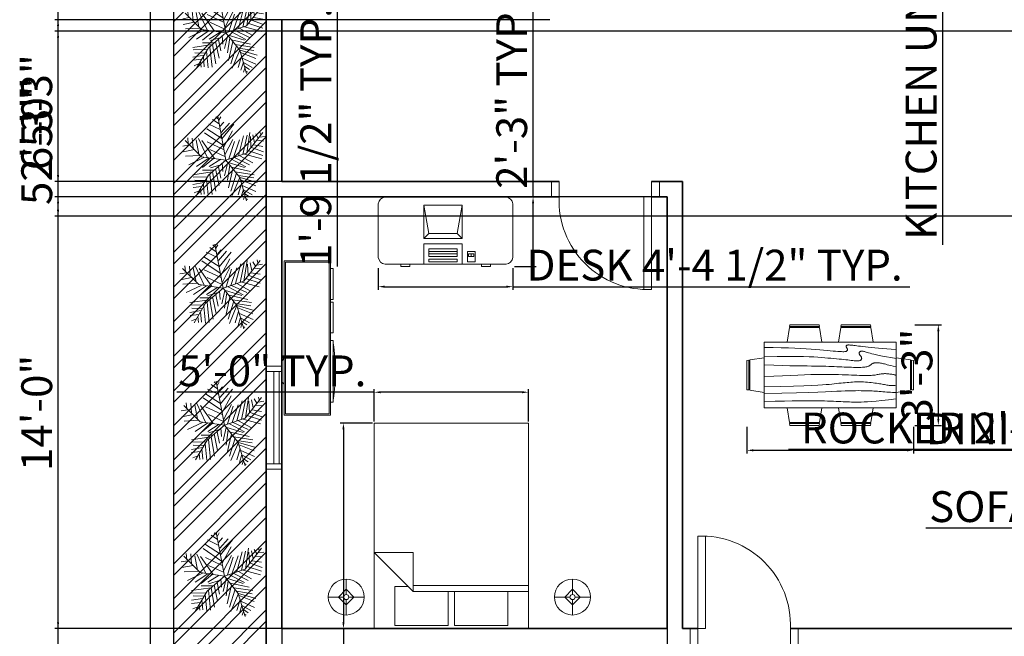
# Model space of a CAD drawing. Units: inches. Extents: x 2297 to 3143, y 440 to 1351.
# Tile 2 of 6: x 2342 to 2725, y 704 to 944. Entities that reach past the tile are written whole.
import ezdxf

# ---------------------------------------------------------------- set-up
doc = ezdxf.new("R2010")
doc.units = ezdxf.units.IN
for name, color, linetype, lineweight in [('A-ANNO-DIMS', 2, 'Continuous', 18), ('A-DOOR', 4, 'Continuous', 20), ('A-EQPM', 8, 'Continuous', 18), ('A-FURN', 8, 'Continuous', 18), ('A-GLAZ', 4, 'Continuous', 18), ('A-WALL', 7, 'Continuous', 35), ('C-PROP', 7, 'Continuous', 25), ('C-SITE-PATT', 252, 'Continuous', 13), ('E-LITE', 9, 'Continuous', 13), ('L-PLNT', 3, 'Continuous', 13)]:
    doc.layers.add(name, color=color, linetype=linetype, lineweight=lineweight)
doc.styles.get("Standard").update_dxf_attribs({"font": 'arial.ttf'})
doc.dimstyles.new('ISO-25', dxfattribs={"dimtxt": 12, "dimasz": 2.5, "dimexe": 1.25, "dimexo": 0.625, "dimtad": 1, "dimdec": 1, "dimlunit": 3, "dimtxsty": 'Standard', "dimcen": 2.5, "dimadec": 0, "dimazin": 0, "dimtfac": 1, "dimtdec": 1, "dimtmove": 0, "dimatfit": 3, "dimfxl": 1, "dimarcsym": 0})

# ---------------------------------------------------------------- blocks, each defined once
blk = doc.blocks.new('Dining Set - 36 x 72 in.')
for p, q in [((-22, 27.5), (-22.1562, 26.50042)), ((-22, 27.5), (-6, 27.5)), ((-5.8437, 26.49966), (-6, 27.5)), ((6, 27.5), (5.8438, 26.50042)), ((6, 27.5), (22, 27.5)), ((22.1563, 26.49966), (22, 27.5)), ((-22.2343, 26.00059), (-23.4847, 17.99762)), ((-22.2304, 26), (-5.7608, 26)), ((-5.8416, 26.5), (-22.1534, 26.5)), ((-4.5152, 17.99762), (-5.7655, 25.99926)), ((5.7657, 26.00059), (4.5153, 17.99762)), ((5.7696, 26), (22.2392, 26)), ((22.1584, 26.5), (5.8466, 26.5)), ((23.4848, 17.99762), (22.2345, 25.99926)), ((36, 18), (-36, 18)), ((-36, 18), (-36, -18)), ((36, -18), (36, 18)), ((-45.5, 8), (-44.5004, 8.15617)), ((-45.5, 8), (-45.5, -8)), ((-44.5, -8.15843), (-44.5, 8.15338)), ((-44.0006, 8.23428), (-35.9976, 9.48474)), ((-44, 8.23041), (-44, -8.23915)), ((44.0006, 8.23428), (35.9976, 9.48474)), ((44, 8.23041), (44, -8.23915)), ((44.5, -8.15843), (44.5, 8.15338)), ((45.5, 8), (44.5005, 8.15617)), ((45.5, 8), (45.5, -8)), ((-44.4997, -8.15631), (-45.5, -8)), ((-35.9976, -9.48476), (-43.9993, -8.2345)), ((35.9976, -9.48476), (43.9993, -8.2345)), ((44.4997, -8.15631), (45.5, -8)), ((-36, -18), (36, -18)), ((-22.2343, -26.0006), (-23.4847, -17.99762)), ((-4.5152, -17.99762), (-5.7655, -25.99928)), ((5.7657, -26.0006), (4.5153, -17.99762)), ((23.4848, -17.99762), (22.2345, -25.99928)), ((-22.2304, -26), (-5.7608, -26)), ((-22, -27.5), (-22.1562, -26.50044)), ((-5.8416, -26.5), (-22.1534, -26.5)), ((-5.8437, -26.49967), (-6, -27.5)), ((5.7696, -26), (22.2392, -26)), ((6, -27.5), (5.8438, -26.50044)), ((22.1584, -26.5), (5.8466, -26.5)), ((22.1563, -26.49967), (22, -27.5)), ((-22, -27.5), (-6, -27.5)), ((6, -27.5), (22, -27.5))]:
    blk.add_line(p, q)
for points in [[(-36, 15), (-31.1772, 14.97754), (-26.8079, 14.91406), (-22.8538, 14.81543), (-19.276, 14.6875), (-16.0362, 14.53613), (-13.0957, 14.36718), (-10.4159, 14.18652), (-7.9583, 14), (-5.6904, 13.81315), (-3.6035, 13.63021), (-1.6954, 13.45508), (0.0365, 13.29166), (1.5945, 13.14388), (2.9811, 13.01562), (4.1988, 12.9108), (5.25, 12.83333), (6.1393, 12.78613), (6.8802, 12.76823), (7.4883, 12.77767), (7.9792, 12.8125), (8.3685, 12.87077), (8.6719, 12.95052), (8.9049, 13.0498), (9.0833, 13.16666), (9.2205, 13.29899), (9.3216, 13.44401), (9.3895, 13.59879), (9.4271, 13.76041), (9.4373, 13.92594), (9.4232, 14.09245), (9.3875, 14.257), (9.3333, 14.41666), (9.2638, 14.56917), (9.1836, 14.71484), (9.0975, 14.85465), (9.0104, 14.98958), (8.9272, 15.1206), (8.8529, 15.2487), (8.7922, 15.37483), (8.75, 15.5), (8.7305, 15.62467), (8.7344, 15.74739), (8.7617, 15.86621), (8.8125, 15.97916), (8.8867, 16.08431), (8.9844, 16.17968), (9.1055, 16.26334), (9.25, 16.33333), (9.4189, 16.38802), (9.6172, 16.42708), (9.8506, 16.45052), (10.125, 16.45833), (10.4463, 16.45052), (10.8203, 16.42708), (11.2529, 16.38802), (11.75, 16.33333), (12.3184, 16.26318), (12.9694, 16.17838), (13.7151, 16.07991), (14.5677, 15.96875), (15.5395, 15.84586), (16.6426, 15.71224), (17.8893, 15.56884), (19.2917, 15.41666), (20.859, 15.25667), (22.5879, 15.08984), (24.4721, 14.91715), (26.5052, 14.73958), (28.6809, 14.5581), (30.9929, 14.3737), (33.4347, 14.18733), (36, 14)], [(-36, 10), (-28.9766, 10.14274), (-23.1725, 10.20442), (-18.4241, 10.19775), (-14.5677, 10.13541), (-11.4399, 10.03011), (-8.877, 9.89453), (-6.7154, 9.74137), (-4.7917, 9.58333), (-2.9698, 9.43082), (-1.2246, 9.28515), (0.4415, 9.14534), (2.026, 9.01041), (3.5266, 8.87939), (4.9408, 8.7513), (6.266, 8.62516), (7.5, 8.5), (8.6411, 8.37549), (9.6914, 8.2539), (10.6538, 8.13818), (11.5312, 8.03125), (12.3267, 7.93603), (13.043, 7.85547), (13.6831, 7.79248), (14.25, 7.75), (14.7471, 7.7303), (15.1797, 7.73307), (15.5537, 7.75732), (15.875, 7.80208), (16.1494, 7.86637), (16.3828, 7.94922), (16.5811, 8.04964), (16.75, 8.16666), (16.8944, 8.29915), (17.0143, 8.44531), (17.1089, 8.60319), (17.1771, 8.77083), (17.218, 8.94629), (17.2305, 9.1276), (17.2137, 9.31282), (17.1667, 9.5), (17.0895, 9.6875), (16.987, 9.875), (16.8649, 10.0625), (16.7292, 10.25), (16.5856, 10.4375), (16.4401, 10.625), (16.2985, 10.8125), (16.1667, 11), (16.05, 11.18733), (15.9518, 11.3737), (15.8752, 11.5581), (15.8229, 11.73958), (15.798, 11.91715), (15.8034, 12.08984), (15.842, 12.25667), (15.9167, 12.41666), (16.0295, 12.56836), (16.1784, 12.70833), (16.3605, 12.83268), (16.5729, 12.9375), (16.8127, 13.01888), (17.0768, 13.07291), (17.3625, 13.0957), (17.6667, 13.08333), (17.9894, 13.03312), (18.3418, 12.94726), (18.7382, 12.82918), (19.1927, 12.68229), (19.7195, 12.51001), (20.3327, 12.31575), (21.0465, 12.10294), (21.875, 11.875), (22.8357, 11.63354), (23.959, 11.37304), (25.2786, 11.08618), (26.8282, 10.76562), (28.6414, 10.40405), (30.752, 9.99414), (33.1936, 9.52856), (36, 9)], [(-36, 5.5), (-30.7157, 5.3348), (-26.069, 5.20963), (-21.9946, 5.11767), (-18.4271, 5.05208), (-15.3009, 5.00602), (-12.5508, 4.97265), (-10.1112, 4.94515), (-7.9167, 4.91666), (-5.909, 4.88167), (-4.0586, 4.83984), (-2.3429, 4.79215), (-0.7396, 4.73958), (0.7739, 4.6831), (2.22, 4.6237), (3.6213, 4.56233), (5, 4.5), (6.373, 4.43782), (7.7344, 4.3776), (9.0723, 4.32129), (10.375, 4.27083), (11.6309, 4.22819), (12.8281, 4.19531), (13.9551, 4.17415), (15, 4.16666), (15.954, 4.17448), (16.819, 4.19791), (17.6001, 4.23698), (18.3021, 4.29166), (18.9299, 4.36198), (19.4883, 4.44791), (19.9823, 4.54948), (20.4167, 4.66666), (20.7969, 4.79899), (21.1302, 4.94401), (21.4245, 5.09879), (21.6875, 5.26041), (21.9271, 5.42594), (22.1511, 5.59245), (22.3672, 5.757), (22.5834, 5.91666), (22.8065, 6.06868), (23.0404, 6.21093), (23.2879, 6.34147), (23.5521, 6.45833), (23.8358, 6.55957), (24.142, 6.64323), (24.4735, 6.70735), (24.8334, 6.75), (25.2235, 6.76969), (25.642, 6.76692), (26.0858, 6.74267), (26.5521, 6.69791), (27.0379, 6.63362), (27.5404, 6.55078), (28.0565, 6.45036), (28.5834, 6.33333), (29.1242, 6.19987), (29.7071, 6.04687), (30.3661, 5.87044), (31.1354, 5.66666), (32.0493, 5.43164), (33.142, 5.16146), (34.4475, 4.85221), (36, 4.5)], [(-36, -1), (-30.7915, -0.6591), (-26.0195, -0.38216), (-21.6519, -0.16284), (-17.6563, 0.00521), (-14.0005, 0.12833), (-10.6523, 0.21289), (-7.5796, 0.26522), (-4.75, 0.29166), (-2.134, 0.29793), (0.2878, 0.28711), (2.5317, 0.26163), (4.6146, 0.22396), (6.5529, 0.17651), (8.3633, 0.12174), (10.0623, 0.06209), (11.6667, 0), (13.1899, -0.06201), (14.6341, -0.1211), (15.9982, -0.17432), (17.2813, -0.21875), (18.4823, -0.25147), (19.6003, -0.26953), (20.6343, -0.27002), (21.5834, -0.25), (22.4481, -0.20768), (23.2357, -0.14584), (23.9549, -0.06836), (24.6146, 0.02083), (25.2235, 0.11784), (25.7904, 0.21875), (26.3241, 0.31966), (26.8334, 0.41666), (27.3265, 0.50618), (27.8099, 0.58593), (28.2894, 0.65397), (28.7709, 0.70833), (29.2601, 0.74707), (29.763, 0.76823), (30.2855, 0.76985), (30.8334, 0.75), (31.4088, 0.70784), (31.9994, 0.64713), (32.589, 0.57275), (33.1615, 0.48958), (33.7008, 0.4025), (34.1908, 0.3164), (34.6153, 0.23616), (34.9584, 0.16666), (35.2099, 0.11165), (35.3848, 0.07031), (35.504, 0.04069), (35.5886, 0.02083), (35.6594, 0.00879), (35.7377, 0.0026), (35.8442, 0.00032), (36, 0)], [(-36, -6.5), (-27.1843, -6.31267), (-20.084, -6.1263), (-14.469, -5.9419), (-10.1094, -5.76042), (-6.7752, -5.58285), (-4.2363, -5.41016), (-2.2629, -5.24333), (-0.625, -5.08334), (0.8708, -4.93099), (2.2715, -4.78646), (3.5872, -4.64974), (4.8281, -4.52084), (6.0046, -4.39974), (7.127, -4.28646), (8.2053, -4.18099), (9.25, -4.08334), (10.2705, -3.99382), (11.2734, -3.91407), (12.2647, -3.84603), (13.25, -3.79167), (14.2354, -3.75293), (15.2266, -3.73177), (16.2295, -3.73015), (17.25, -3.75), (18.2912, -3.79248), (19.3451, -3.85547), (20.4009, -3.93604), (21.4479, -4.03125), (22.4754, -4.13819), (23.4727, -4.25391), (24.4289, -4.37549), (25.3334, -4.5), (26.1785, -4.62492), (26.9694, -4.74935), (27.7145, -4.87281), (28.4219, -4.99479), (29.1, -5.11483), (29.7572, -5.23242), (30.4016, -5.34709), (31.0417, -5.45834), (31.6837, -5.56437), (32.3262, -5.65821), (32.9658, -5.73153), (33.599, -5.77604), (34.2224, -5.78345), (34.8327, -5.74545), (35.4264, -5.65373), (36, -5.5)], [(-36, -10), (-26.4022, -9.81299), (-18.4675, -9.62891), (-11.9839, -9.45069), (-6.7396, -9.28125), (-2.5226, -9.12354), (0.8789, -8.98047), (3.6769, -8.85498), (6.0833, -8.75), (8.2767, -8.66765), (10.3021, -8.60677), (12.1712, -8.56543), (13.8958, -8.54167), (15.4876, -8.53353), (16.9583, -8.53907), (18.3197, -8.55632), (19.5834, -8.58334), (20.7616, -8.61841), (21.8685, -8.66081), (22.9188, -8.71004), (23.9271, -8.76563), (24.9081, -8.82707), (25.8763, -8.89388), (26.8465, -8.96558), (27.8334, -9.04167), (28.8474, -9.12118), (29.8828, -9.20117), (30.93, -9.27824), (31.9792, -9.34896), (33.0205, -9.40991), (34.0443, -9.45768), (35.0407, -9.48885), (36, -9.5)], [(-36, -14.5), (-30.0881, -14.33513), (-25.0332, -14.21224), (-20.7312, -14.12647), (-17.0781, -14.07292), (-13.97, -14.04671), (-11.3027, -14.04297), (-8.9724, -14.05681), (-6.875, -14.08334), (-4.9224, -14.11833), (-3.0905, -14.16016), (-1.3709, -14.20785), (0.2448, -14.26042), (1.7647, -14.3169), (3.1973, -14.3763), (4.5507, -14.43767), (5.8333, -14.5), (7.0554, -14.5621), (8.235, -14.62175), (9.3922, -14.67652), (10.5469, -14.72396), (11.7192, -14.76164), (12.929, -14.78711), (14.1965, -14.79794), (15.5417, -14.79167), (16.9933, -14.76424), (18.6152, -14.70508), (20.4804, -14.60197), (22.6615, -14.44271), (25.2312, -14.21509), (28.2624, -13.9069), (31.8277, -13.50594), (36, -13)]]:
    blk.add_lwpolyline(points)
blk = doc.blocks.new('Bed - Queen')
for p, q in [((0, -80.00003), (0, 0)), ((0, 0), (59.99999, 0)), ((59.99999, 0), (59.99999, -80.00003)), ((7.99999, -1.2), (28.79998, -1.2)), ((7.99999, -14.4), (7.99999, -1.2)), ((28.79998, -1.2), (28.79998, -14.4)), ((31.19999, -1.2), (51.99999, -1.2)), ((31.19999, -14.4), (31.19999, -1.2)), ((51.99999, -1.2), (51.99999, -16.4)), ((0, -14.4), (44.8, -14.4)), ((59.99999, -29.6), (44.8, -14.4)), ((44.8, -14.4), (44.8, -29.6)), ((44.8, -16.8), (0, -16.8)), ((51.99999, -16.4), (46.79936, -16.4)), ((44.8, -29.6), (59.99999, -29.6)), ((59.99999, -80.00003), (0, -80.00003))]:
    blk.add_line(p, q)
blk = doc.blocks.new('*U16')
for p, q in [((-8.737, 47.138), (-17.069, 52.711)), ((-10.186, 53.64), (-13.084, 55.962)), ((0, 0), (-10.5, 57)), ((-9.099, 51.782), (-6.563, 55.962)), ((-5.114, 28.097), (-24.676, 40.636)), ((-7.288, 39.707), (-21.778, 46.673)), ((-7.65, 43.423), (-2.578, 49.46)), ((-5.839, 35.992), (4.667, 48.067)), ((-5.114, 27.632), (10.463, 46.673)), ((-48.585, 21.131), (-49.309, 29.026)), ((-43.513, 28.561), (-42.427, 15.558)), ((-38.442, 26.239), (-34.819, 7.663)), ((-35.544, 28.097), (-24.314, 3.947)), ((-3.665, 19.273), (-27.574, 35.527)), ((-2.941, 16.486), (8.652, 37.85)), ((-1.129, 6.734), (9.014, 26.704)), ((10.101, 3.483), (17.708, 26.239)), ((16.259, 5.805), (23.142, 31.348)), ((22.055, 7.198), (27.489, 32.277)), ((27, 9), (48, 36)), ((27.127, 9.056), (31.112, 35.992)), ((31.836, 30.883), (32.561, 16.486)), ((35.096, 32.741), (37.27, 22.524)), ((38.719, 34.134), (41.979, 28.561)), ((40.53, 25.775), (48.862, 24.846)), ((43.791, 29.954), (51.036, 30.883)), ((44.153, 36.456), (45.239, 32.741)), ((-47.498, 19.737), (-55.83, 18.344)), ((-40.615, 13.7), (-55.105, 10.913)), ((-31.5, 4.5), (-52.5, 25.5)), ((-14.533, 2.09), (-30.834, 25.31)), ((-24.314, 23.917), (-2.941, 13.7)), ((-20.691, 13.7), (-1.129, 4.876)), ((3.942, 1.625), (11.187, 24.381)), ((33.285, 16.486), (48.862, 10.913)), ((36.183, 19.737), (48.137, 17.88)), ((-33.37, 6.269), (-52.207, 5.34)), ((-28.299, 3.483), (-47.86, -5.805)), ((-21.416, 3.018), (-38.079, -8.128)), ((0, 0), (-31.5, 4.5)), ((-15.982, 2.09), (-30.11, -9.521)), ((0, 0), (-22.5, -19.5)), ((-6.563, 1.161), (-21.416, -8.128)), ((0, 0), (27, 9)), ((0, 0), (18, -22.5)), ((6.478, 1.625), (26.04, -8.592)), ((11.187, 3.483), (30.749, -5.805)), ((18.07, 5.805), (35.096, -3.483)), ((24.229, 7.663), (46.688, 1.625)), ((29.662, 12.307), (48.137, 6.269)), ((-6.563, -5.805), (-19.967, -9.985)), ((-13.446, -11.378), (-8.737, -32.741)), ((-9.461, -8.592), (-6.201, -23.453)), ((-4.752, -3.483), (-3.665, -14.629)), ((2.493, -3.019), (-1.491, -20.202)), ((1.769, -2.555), (24.229, -9.521)), ((5.029, -6.27), (2.131, -25.775)), ((9.014, -11.378), (3.58, -35.992)), ((7.565, -9.056), (32.198, -14.629)), ((-17.431, -15.094), (-42.789, -18.809)), ((-24.314, -21.596), (-42.427, -22.06)), ((-22.5, -19.5), (-37.5, -45)), ((-15.257, -12.772), (-30.11, -12.772)), ((-25.038, -23.918), (-22.865, -45.281)), ((-20.691, -18.345), (-17.793, -44.352)), ((-17.069, -15.094), (-12.721, -40.172)), ((14.085, -16.951), (6.478, -40.172)), ((18.07, -22.524), (8.289, -45.745)), ((12.274, -15.094), (36.907, -18.809)), ((16.259, -19.738), (36.183, -22.989)), ((18, -22.5), (27, -52.5)), ((18.433, -22.524), (40.53, -29.026)), ((19.157, -25.311), (38.719, -33.206)), ((-28.299, -29.026), (-42.789, -31.348)), ((-30.834, -34.135), (-42.427, -35.528)), ((-26.849, -26.24), (-40.253, -25.775)), ((-32.646, -36.921), (-31.921, -44.352)), ((-29.023, -30.884), (-27.936, -43.887)), ((20.244, -30.419), (15.897, -44.816)), ((22.78, -37.85), (19.519, -48.532)), ((21.331, -32.741), (39.081, -40.636)), ((-34.457, -39.708), (-40.978, -42.494)), ((22.78, -38.314), (34.372, -44.816)), ((24.591, -45.745), (23.142, -50.854)), ((24.591, -43.423), (30.749, -47.603)), ((26.764, -49.925), (28.213, -50.854))]:
    blk.add_line(p, q)
blk = doc.blocks.new('Lamp - Table')
for p, q in [((0, 7), (0, 1)), ((-1, 0), (-7, 0)), ((0, 3), (-3, 0)), ((-3, 0), (0, -3)), ((3, 0), (0, 3)), ((0, -3), (3, 0)), ((1, 0), (7, 0)), ((0, -1), (0, -7))]:
    blk.add_line(p, q)
for radius in [7, 1]:
    blk.add_circle((0, 0), radius)
blk = doc.blocks.new('Desk - 30 x 60 in.')
for p, q in [((-26.999995, 0), (26.999995, 0)), ((-29.999995, -27), (-29.999995, -3)), ((29.999995, -3), (29.999995, -27)), ((26.999995, -30), (-26.999995, -30)), ((-20.000005, -30), (-20.000005, -31)), ((-16.000005, -31), (-16.000005, -30)), ((15.999995, -31), (15.999995, -30)), ((19.999995, -30), (19.999995, -31)), ((-20.000005, -31), (-16.000005, -31)), ((19.999995, -31), (15.999995, -31))]:
    blk.add_line(p, q)
for centre, start, end in [((-26.499995, -3.5), 98.1301, 171.8699), ((26.499995, -3.5), 8.130102, 81.8699), ((-26.499995, -26.5), 188.1301, 261.8699), ((26.499995, -26.5), 278.1301, 351.8699)]:
    blk.add_arc(centre, 3.535534, start, end)
blk = doc.blocks.new('Computer Terminal')
for p, q in [((-10, 11.5), (5, 11.5)), ((-8, 0.5), (-10, 11.5)), ((-10, -1.5), (-10, 11.5)), ((5, 11.5), (3, 0.5)), ((5, 11.5), (5, -1.5)), ((-10, -1.5), (-8, 0.5)), ((3, 0.5), (-8, 0.5)), ((3, 0.5), (5, -1.5)), ((5, -1.5), (-10, -1.5)), ((-10, -11.5), (-10, -3.5)), ((-10, -3.5), (5, -3.5)), ((5, -3.5), (5, -11.5)), ((-8, -5.5), (-8, -8.5)), ((3, -5.5), (-8, -5.5)), ((3, -6.5), (-8, -6.5)), ((-8, -7.5), (3, -7.5)), ((3, -8.5), (3, -5.5)), ((10, -6.5), (7, -6.5)), ((7, -6.5), (7, -10.5)), ((9.5, -7.5), (7.5, -7.5)), ((7.5, -7.5), (7.5, -8.5)), ((8.5, -7.5), (8.5, -8.5)), ((9.5, -8.5), (9.5, -7.5)), ((10, -10.5), (10, -6.5)), ((-8, -8.5), (3, -8.5)), ((-8, -9.5), (-8, -10.5)), ((3, -9.5), (-8, -9.5)), ((-8, -10.5), (3, -10.5)), ((3, -10.5), (3, -9.5)), ((7, -10.5), (10, -10.5)), ((7.5, -8.5), (9.5, -8.5)), ((5, -11.5), (-10, -11.5))]:
    blk.add_line(p, q)
blk = doc.blocks.new('Entertainment Center')
for p, q in [((-4, 0), (-5, -1)), ((4, 0), (-4, 0)), ((5, -1), (4, 0)), ((-17, -19), (-17, -1)), ((-17, -1), (43, -1)), ((-16.5, -18.5), (-16.5, -1.5)), ((-16.5, -1.5), (42.5, -1.5)), ((42.5, -1.5), (42.5, -18.5)), ((43, -1), (43, -19)), ((43, -19), (-17, -19)), ((42.5, -18.5), (-16.5, -18.5)), ((-12, -20), (-12, -19)), ((12, -19), (12, -20)), ((15, -20), (15, -19)), ((27, -19), (27, -20)), ((28, -20), (28, -19)), ((40, -19), (40, -20)), ((12, -20), (-12, -20)), ((27, -20), (15, -20)), ((40, -20), (28, -20))]:
    blk.add_line(p, q)
blk.add_arc((0, 40), 61, 259.6111, 280.3889)
blk = doc.blocks.new('DOOR-36IN-6IN-JAMB')
for p, q in [((0, 6), (0, 0)), ((3, 6), (3, 0)), ((39, 6), (39, 0)), ((42, 6), (42, 0))]:
    blk.add_line(p, q)
blk.add_lwpolyline([(39, 6), (36, 6), (36, 42), (39, 42)], close=True)
blk.add_arc((37.5, 7.5), 34.53, 87.5104, 182.4896)
blk = doc.blocks.new('WIN-36IN-6IN-WALL')
for p, q in [((6, 40), (0, 40)), ((6, 38), (0, 38)), ((3, 38), (3, 2)), ((5, 38), (5, 2)), ((0, 2), (6, 2)), ((0, 0), (6, 0))]:
    blk.add_line(p, q)
blk = doc.blocks.new('*D33')
at = {"layer": 'A-ANNO-DIMS', "color": 0, "lineweight": -2, "transparency": 16777216}
for p, q in [((2481.79, 846.95), (2481.79, 838.47)), ((2534.17, 846.95), (2534.17, 838.47)), ((2484.29, 839.72), (2531.67, 839.72)), ((2534.17, 839.72), (2688.74, 839.72))]:
    blk.add_line(p, q, dxfattribs=at)
at = {"layer": 'A-ANNO-DIMS', "color": 0, "transparency": 16777216}
for points in [[(2484.29, 840.13), (2484.29, 839.3), (2481.79, 839.72)], [(2531.67, 840.13), (2531.67, 839.3), (2534.17, 839.72)]]:
    blk.add_solid(points, dxfattribs=at)
at = {"layer": 'Defpoints', "color": 0, "transparency": 16777216}
for p in [(2481.79, 847.57), (2534.17, 847.57), (2534.17, 839.72)]:
    blk.add_point(p, dxfattribs=at)
at = {"layer": 'A-ANNO-DIMS', "color": 0, "transparency": 16777216, "insert": (2612.7, 846.55), "char_height": 12, "attachment_point": 5}
blk.add_mtext('DESK 4\'-4 1/2" TYP.', dxfattribs=at)
blk = doc.blocks.new('*D34')
at = {"layer": 'A-ANNO-DIMS', "color": 0, "lineweight": -2, "transparency": 16777216}
for p, q in [((2542.03, 874.63), (2542.03, 951.74)), ((2534.79, 874.63), (2543.28, 874.63)), ((2542.03, 850.07), (2542.03, 872.13)), ((2534.79, 847.57), (2543.28, 847.57))]:
    blk.add_line(p, q, dxfattribs=at)
at = {"layer": 'A-ANNO-DIMS', "color": 0, "transparency": 16777216}
for points in [[(2541.61, 872.13), (2542.44, 872.13), (2542.03, 874.63)], [(2541.61, 850.07), (2542.44, 850.07), (2542.03, 847.57)]]:
    blk.add_solid(points, dxfattribs=at)
at = {"layer": 'Defpoints', "color": 0, "transparency": 16777216}
for p in [(2534.17, 874.63), (2542.03, 874.63), (2534.17, 847.57)]:
    blk.add_point(p, dxfattribs=at)
at = {"layer": 'A-ANNO-DIMS', "color": 0, "transparency": 16777216, "insert": (2535.27, 914.43), "char_height": 12, "attachment_point": 5, "rotation": 90}
blk.add_mtext('2\'-3" TYP.', dxfattribs=at)
blk = doc.blocks.new('*D37')
at = {"layer": 'A-ANNO-DIMS', "color": 0, "lineweight": -2, "transparency": 16777216}
for p, q in [((2479.6, 786.63), (2466.97, 786.63)), ((2468.22, 784.13), (2468.22, 709.13)), ((2479.6, 706.63), (2466.97, 706.63)), ((2468.22, 706.63), (2468.22, 526.36))]:
    blk.add_line(p, q, dxfattribs=at)
at = {"layer": 'A-ANNO-DIMS', "color": 0, "transparency": 16777216}
for points in [[(2467.8, 784.13), (2468.64, 784.13), (2468.22, 786.63)], [(2467.8, 709.13), (2468.64, 709.13), (2468.22, 706.63)]]:
    blk.add_solid(points, dxfattribs=at)
at = {"layer": 'Defpoints', "color": 0, "transparency": 16777216}
for p in [(2480.22, 786.63), (2468.22, 706.63), (2480.22, 706.63)]:
    blk.add_point(p, dxfattribs=at)
at = {"layer": 'A-ANNO-DIMS', "color": 0, "transparency": 16777216, "insert": (2461.02, 615.25), "char_height": 12, "attachment_point": 5, "rotation": 90}
blk.add_mtext('QUEEN BED 6\'-8" TYP.', dxfattribs=at)
blk = doc.blocks.new('*D38')
at = {"layer": 'A-ANNO-DIMS', "color": 0, "lineweight": -2, "transparency": 16777216}
for p, q in [((2480.22, 798.63), (2403.32, 798.63)), ((2480.22, 787.26), (2480.22, 799.88)), ((2537.72, 798.63), (2482.72, 798.63)), ((2540.22, 787.26), (2540.22, 799.88))]:
    blk.add_line(p, q, dxfattribs=at)
at = {"layer": 'A-ANNO-DIMS', "color": 0, "transparency": 16777216}
for points in [[(2482.72, 799.05), (2482.72, 798.22), (2480.22, 798.63)], [(2537.72, 799.05), (2537.72, 798.22), (2540.22, 798.63)]]:
    blk.add_solid(points, dxfattribs=at)
at = {"layer": 'Defpoints', "color": 0, "transparency": 16777216}
for p in [(2480.22, 798.63), (2480.22, 786.63), (2540.22, 786.63)]:
    blk.add_point(p, dxfattribs=at)
at = {"layer": 'A-ANNO-DIMS', "color": 0, "transparency": 16777216, "insert": (2440.52, 805.39), "char_height": 12, "attachment_point": 5}
blk.add_mtext('5\'-0" TYP.', dxfattribs=at)
blk = doc.blocks.new('*D42')
at = {"layer": 'A-ANNO-DIMS', "color": 0, "lineweight": -2, "transparency": 16777216}
for p, q in [((2474.21, 972.57), (2464.59, 972.57)), ((2465.84, 970.07), (2465.84, 953.74)), ((2474.21, 951.24), (2464.59, 951.24)), ((2465.84, 951.24), (2465.84, 847.51))]:
    blk.add_line(p, q, dxfattribs=at)
at = {"layer": 'A-ANNO-DIMS', "color": 0, "transparency": 16777216}
for points in [[(2465.42, 970.07), (2466.25, 970.07), (2465.84, 972.57)], [(2465.42, 953.74), (2466.25, 953.74), (2465.84, 951.24)]]:
    blk.add_solid(points, dxfattribs=at)
at = {"layer": 'Defpoints', "color": 0, "transparency": 16777216}
for p in [(2474.84, 972.57), (2465.84, 951.24), (2474.84, 951.24)]:
    blk.add_point(p, dxfattribs=at)
at = {"layer": 'A-ANNO-DIMS', "color": 0, "transparency": 16777216, "insert": (2459.01, 898.13), "char_height": 12, "attachment_point": 5, "rotation": 90}
blk.add_mtext('1\'-9 1/2" TYP.', dxfattribs=at)
blk = doc.blocks.new('*D49')
at = {"layer": 'A-ANNO-DIMS', "color": 0, "lineweight": -2, "transparency": 16777216}
for p, q in [((2818.08, 745.72), (2694.9, 745.72)), ((2818.08, 735.78), (2818.08, 746.97)), ((2886.03, 745.72), (2820.58, 745.72)), ((2888.53, 735.78), (2888.53, 746.97))]:
    blk.add_line(p, q, dxfattribs=at)
at = {"layer": 'A-ANNO-DIMS', "color": 0, "transparency": 16777216}
for points in [[(2820.58, 746.14), (2820.58, 745.3), (2818.08, 745.72)], [(2886.03, 746.14), (2886.03, 745.3), (2888.53, 745.72)]]:
    blk.add_solid(points, dxfattribs=at)
at = {"layer": 'Defpoints', "color": 0, "transparency": 16777216}
for p in [(2818.08, 745.72), (2818.08, 735.15), (2888.53, 735.15)]:
    blk.add_point(p, dxfattribs=at)
at = {"layer": 'A-ANNO-DIMS', "color": 0, "transparency": 16777216, "insert": (2755.24, 752.55), "char_height": 12, "attachment_point": 5}
blk.add_mtext('SOFA 5\'-10 1/2"', dxfattribs=at)
blk = doc.blocks.new('*D53')
at = {"layer": 'A-ANNO-DIMS', "color": 0, "lineweight": -2, "transparency": 16777216}
for p, q in [((2794.15, 776.31), (2641.5, 776.31)), ((2794.15, 772.88), (2794.15, 777.56)), ((2818.65, 776.31), (2796.65, 776.31)), ((2821.15, 772.88), (2821.15, 777.56))]:
    blk.add_line(p, q, dxfattribs=at)
at = {"layer": 'A-ANNO-DIMS', "color": 0, "transparency": 16777216}
for points in [[(2796.65, 776.72), (2796.65, 775.89), (2794.15, 776.31)], [(2818.65, 776.72), (2818.65, 775.89), (2821.15, 776.31)]]:
    blk.add_solid(points, dxfattribs=at)
at = {"layer": 'Defpoints', "color": 0, "transparency": 16777216}
for p in [(2794.15, 776.31), (2794.15, 772.26), (2821.15, 772.26)]:
    blk.add_point(p, dxfattribs=at)
at = {"layer": 'A-ANNO-DIMS', "color": 0, "transparency": 16777216, "insert": (2716.58, 783.14), "char_height": 12, "attachment_point": 5}
blk.add_mtext('ROCKER 2\'-3" TYP.', dxfattribs=at)
blk = doc.blocks.new('*D61')
at = {"layer": 'A-ANNO-DIMS', "color": 0, "lineweight": -2, "transparency": 16777216}
for p, q in [((2710.47, 1077.25), (2700.22, 1077.25)), ((2701.47, 1074.75), (2701.47, 1015.6)), ((2710.47, 1013.1), (2700.22, 1013.1)), ((2701.47, 1013.1), (2701.47, 855.98))]:
    blk.add_line(p, q, dxfattribs=at)
at = {"layer": 'A-ANNO-DIMS', "color": 0, "transparency": 16777216}
for points in [[(2701.05, 1074.75), (2701.89, 1074.75), (2701.47, 1077.25)], [(2701.05, 1015.6), (2701.89, 1015.6), (2701.47, 1013.1)]]:
    blk.add_solid(points, dxfattribs=at)
at = {"layer": 'Defpoints', "color": 0, "transparency": 16777216}
for p in [(2711.09, 1077.25), (2701.47, 1013.1), (2711.09, 1013.1)]:
    blk.add_point(p, dxfattribs=at)
at = {"layer": 'A-ANNO-DIMS', "color": 0, "transparency": 16777216, "insert": (2694.64, 933.29), "char_height": 12, "attachment_point": 5, "rotation": 90}
blk.add_mtext('KITCHEN UNIT 5\'-4"', dxfattribs=at)
blk = doc.blocks.new('*D63')
at = {"layer": 'A-ANNO-DIMS', "color": 0, "lineweight": -2, "transparency": 16777216}
for p, q in [((2625.28, 785.11), (2625.28, 774.77)), ((2690.07, 785.11), (2690.07, 774.77)), ((2627.78, 776.02), (2687.57, 776.02)), ((2690.07, 776.02), (2825.72, 776.02))]:
    blk.add_line(p, q, dxfattribs=at)
at = {"layer": 'A-ANNO-DIMS', "color": 0, "transparency": 16777216}
for points in [[(2627.78, 776.44), (2627.78, 775.6), (2625.28, 776.02)], [(2687.57, 776.44), (2687.57, 775.6), (2690.07, 776.02)]]:
    blk.add_solid(points, dxfattribs=at)
at = {"layer": 'Defpoints', "color": 0, "transparency": 16777216}
for p in [(2625.28, 785.74), (2690.07, 785.74), (2690.07, 776.02)]:
    blk.add_point(p, dxfattribs=at)
at = {"layer": 'A-ANNO-DIMS', "color": 0, "transparency": 16777216, "insert": (2759.14, 782.85), "char_height": 12, "attachment_point": 5}
blk.add_mtext('DINING SET 5\'-5"', dxfattribs=at)
blk = doc.blocks.new('*D64')
at = {"layer": 'A-ANNO-DIMS', "color": 0, "lineweight": -2, "transparency": 16777216}
for p, q in [((2690.7, 824.9), (2701.04, 824.9)), ((2699.79, 788.24), (2699.79, 822.4)), ((2690.7, 785.74), (2701.04, 785.74))]:
    blk.add_line(p, q, dxfattribs=at)
at = {"layer": 'A-ANNO-DIMS', "color": 0, "transparency": 16777216}
for points in [[(2699.37, 822.4), (2700.21, 822.4), (2699.79, 824.9)], [(2699.37, 788.24), (2700.21, 788.24), (2699.79, 785.74)]]:
    blk.add_solid(points, dxfattribs=at)
at = {"layer": 'Defpoints', "color": 0, "transparency": 16777216}
for p in [(2690.07, 824.9), (2699.79, 824.9), (2690.07, 785.74)]:
    blk.add_point(p, dxfattribs=at)
at = {"layer": 'A-ANNO-DIMS', "color": 0, "transparency": 16777216, "insert": (2693.03, 805.32), "char_height": 12, "attachment_point": 5, "rotation": 90}
blk.add_mtext('3\'-3"', dxfattribs=at)
blk = doc.blocks.new('*D70')
at = {"layer": 'A-ANNO-DIMS', "color": 0, "lineweight": -2, "transparency": 16777216}
for p, q in [((2392.57, 1207.63), (2355.89, 1207.63)), ((2357.14, 583.13), (2357.14, 1205.13)), ((2437.57, 580.63), (2355.89, 580.63))]:
    blk.add_line(p, q, dxfattribs=at)
at = {"layer": 'A-ANNO-DIMS', "color": 0, "transparency": 16777216}
for points in [[(2356.73, 1205.13), (2357.56, 1205.13), (2357.14, 1207.63)], [(2356.73, 583.13), (2357.56, 583.13), (2357.14, 580.63)]]:
    blk.add_solid(points, dxfattribs=at)
at = {"layer": 'Defpoints', "color": 0, "transparency": 16777216}
for p in [(2357.14, 1207.63), (2393.19, 1207.63), (2438.19, 580.63)]:
    blk.add_point(p, dxfattribs=at)
at = {"layer": 'A-ANNO-DIMS', "color": 0, "transparency": 16777216, "insert": (2350.39, 894.13), "char_height": 12, "attachment_point": 5, "rotation": 90}
blk.add_mtext('52\'-3"', dxfattribs=at)
blk = doc.blocks.new('*D76')
at = {"layer": 'A-ANNO-DIMS', "color": 0, "lineweight": -2, "transparency": 16777216}
for p, q in [((2593.57, 874.63), (2355.89, 874.63)), ((2357.14, 709.13), (2357.14, 872.13)), ((2593.57, 706.63), (2355.89, 706.63))]:
    blk.add_line(p, q, dxfattribs=at)
at = {"layer": 'A-ANNO-DIMS', "color": 0, "transparency": 16777216}
for points in [[(2356.73, 872.13), (2357.56, 872.13), (2357.14, 874.63)], [(2356.73, 709.13), (2357.56, 709.13), (2357.14, 706.63)]]:
    blk.add_solid(points, dxfattribs=at)
at = {"layer": 'Defpoints', "color": 0, "transparency": 16777216}
for p in [(2357.14, 874.63), (2594.19, 874.63), (2594.19, 706.63)]:
    blk.add_point(p, dxfattribs=at)
at = {"layer": 'A-ANNO-DIMS', "color": 0, "transparency": 16777216, "insert": (2350.39, 790.63), "char_height": 12, "attachment_point": 5, "rotation": 90}
blk.add_mtext('14\'-0"', dxfattribs=at)
blk = doc.blocks.new('*D77')
at = {"layer": 'A-ANNO-DIMS', "color": 0, "lineweight": -2, "transparency": 16777216}
for p, q in [((2444.19, 874.01), (2444.19, 510.33)), ((2594.19, 874.01), (2594.19, 510.33)), ((2446.69, 511.58), (2591.69, 511.58))]:
    blk.add_line(p, q, dxfattribs=at)
at = {"layer": 'A-ANNO-DIMS', "color": 0, "transparency": 16777216}
for points in [[(2446.69, 512), (2446.69, 511.17), (2444.19, 511.58)], [(2591.69, 512), (2591.69, 511.17), (2594.19, 511.58)]]:
    blk.add_solid(points, dxfattribs=at)
at = {"layer": 'Defpoints', "color": 0, "transparency": 16777216}
for p in [(2444.19, 874.63), (2594.19, 874.63), (2594.19, 511.58)]:
    blk.add_point(p, dxfattribs=at)
at = {"layer": 'A-ANNO-DIMS', "color": 0, "transparency": 16777216, "insert": (2519.19, 518.34), "char_height": 12, "attachment_point": 5}
blk.add_mtext('12\'-6"', dxfattribs=at)
blk = doc.blocks.new('*D78')
at = {"layer": 'A-ANNO-DIMS', "color": 0, "lineweight": -2, "transparency": 16777216}
for p, q in [((2548.57, 943.63), (2355.89, 943.63)), ((2357.14, 883.13), (2357.14, 941.13)), ((2548.57, 880.63), (2355.89, 880.63))]:
    blk.add_line(p, q, dxfattribs=at)
at = {"layer": 'A-ANNO-DIMS', "color": 0, "transparency": 16777216}
for points in [[(2356.73, 941.13), (2357.56, 941.13), (2357.14, 943.63)], [(2356.73, 883.13), (2357.56, 883.13), (2357.14, 880.63)]]:
    blk.add_solid(points, dxfattribs=at)
at = {"layer": 'Defpoints', "color": 0, "transparency": 16777216}
for p in [(2357.14, 943.63), (2549.19, 943.63), (2549.19, 880.63)]:
    blk.add_point(p, dxfattribs=at)
at = {"layer": 'A-ANNO-DIMS', "color": 0, "transparency": 16777216, "insert": (2350.39, 912.13), "char_height": 12, "attachment_point": 5, "rotation": 90}
blk.add_mtext('5\'-3"', dxfattribs=at)
blk = doc.blocks.new('*D80')
at = {"layer": 'A-ANNO-DIMS', "color": 0, "lineweight": -2, "transparency": 16777216}
for p, q in [((2805.07, 939.13), (2355.89, 939.13)), ((2357.14, 869.63), (2357.14, 936.63)), ((2805.07, 867.13), (2355.89, 867.13))]:
    blk.add_line(p, q, dxfattribs=at)
at = {"layer": 'A-ANNO-DIMS', "color": 0, "transparency": 16777216}
for points in [[(2356.73, 936.63), (2357.56, 936.63), (2357.14, 939.13)], [(2356.73, 869.63), (2357.56, 869.63), (2357.14, 867.13)]]:
    blk.add_solid(points, dxfattribs=at)
at = {"layer": 'Defpoints', "color": 0, "transparency": 16777216}
for p in [(2357.14, 939.13), (2805.69, 939.13), (2805.69, 867.13)]:
    blk.add_point(p, dxfattribs=at)
at = {"layer": 'A-ANNO-DIMS', "color": 0, "transparency": 16777216, "insert": (2350.39, 903.13), "char_height": 12, "attachment_point": 5, "rotation": 90}
blk.add_mtext('6\'-0"', dxfattribs=at)

msp = doc.modelspace()

# ---------------------------------------------------------------- hatches: boundary and pattern name
at = {"layer": 'C-SITE-PATT'}
h = msp.add_hatch(dxfattribs=at)
h.set_pattern_fill('ANSI32', color=256)
h.paths.add_polyline_path([(2438.19, 1198.63), (2402.19, 1198.63), (2402.19, 556.63), (2667.43, 556.63), (2742.43, 556.63), (2946.69, 556.63), (2982.69, 556.63), (2982.69, 1117.63), (2982.69, 1123.63), (2982.69, 1198.63), (2946.69, 1198.63), (2946.69, 1117.63), (2946.69, 700.63), (2806.19, 700.63), (2806.19, 580.63), (2738.57, 580.63), (2738.57, 589.63), (2735.57, 589.63), (2735.57, 625.63, 0.402069), (2702.6, 591.13, 0.401544), (2669.57, 625.63), (2669.57, 589.63), (2666.57, 589.63), (2666.57, 580.63), (2438.19, 580.63)])
h.paths.add_polyline_path([(2706.46, 558.2, -0.000472), (2706.46, 558.13, -0.000473)], flags=16)
h.paths.add_polyline_path([(2875.15, 576.11), (2920.92, 576.11), (2920.92, 585.31), (2875.15, 585.31)], flags=24)
h.paths.add_polyline_path([(2875.13, 585.74), (2915.96, 585.74), (2915.96, 595.05), (2875.13, 595.05)], flags=24)
h.paths.add_polyline_path([(2646.52, 1069.72), (2687.63, 1069.72), (2687.63, 1078.92), (2646.52, 1078.92)], flags=25)
h.paths.add_polyline_path([(2646.5, 1079.35), (2686.39, 1079.35), (2686.39, 1088.65), (2646.5, 1088.65)], flags=25)

# ---------------------------------------------------------------- linework, layer by layer
at = {"layer": 'A-WALL'}
for p, q in [((2438.19, 580.63), (2438.19, 1198.63)), ((2444.19, 880.63), (2444.19, 943.63)), ((2444.19, 880.63), (2552.19, 880.63)), ((2588.19, 880.63), (2600.19, 880.63)), ((2600.19, 706.63), (2600.19, 880.63)), ((2444.19, 874.63), (2552.19, 874.63)), ((2444.19, 706.63), (2444.19, 874.63)), ((2588.19, 874.63), (2594.19, 874.63)), ((2594.19, 706.63), (2594.19, 874.63)), ((2444.19, 706.63), (2594.19, 706.63)), ((2600.19, 706.63), (2606.19, 706.63)), ((2642.19, 706.63), (2940.69, 706.63))]:
    msp.add_line(p, q, dxfattribs=at)
at = {"layer": 'C-PROP'}
for p, q in [((2393.19, 547.63), (2393.19, 1207.63)), ((2402.19, 556.63), (2402.19, 1198.63))]:
    msp.add_line(p, q, dxfattribs=at)

# ---------------------------------------------------------------- block references
at = {"layer": 'A-DOOR', "extrusion": (0, 0, -1), "zscale": -1, "rotation": 180}
msp.add_blockref('DOOR-36IN-6IN-JAMB', (-2549.19, 880.63), dxfattribs=at)
at = {"layer": 'A-DOOR', "extrusion": (0, 0, -1), "zscale": -1}
msp.add_blockref('DOOR-36IN-6IN-JAMB', (-2645.19, 700.63), dxfattribs=at)
at = {"layer": 'A-EQPM'}
msp.add_blockref('Computer Terminal', (2509.47, 859.95), dxfattribs=at)
at = {"layer": 'A-FURN'}
for name, p, xscale, yscale, zscale in [('Desk - 30 x 60 in.', (2507.98, 874.63), 0.8729228900222988, 0.8729228900222988, 0.8729228900222988), ('Dining Set - 36 x 72 in.', (2657.68, 805.32), 0.7119824199930433, 0.7119824199930433, 0.7119824199930433)]:
    msp.add_blockref(name, p, dxfattribs=dict(at, xscale=xscale, yscale=yscale, zscale=zscale))
for name, p, rotation in [('Entertainment Center', (2444.19, 806.73), 90), ('Bed - Queen', (2540.22, 706.63), 180)]:
    msp.add_blockref(name, p, dxfattribs=dict(at, rotation=rotation))
at = {"layer": 'A-GLAZ'}
msp.add_blockref('WIN-36IN-6IN-WALL', (2438.19, 768.73), dxfattribs=at)
at = {"layer": 'E-LITE'}
for p in [(2469.32, 718.92), (2557.4, 718.92)]:
    msp.add_blockref('Lamp - Table', p, dxfattribs=at)
at = {"layer": 'L-PLNT', "xscale": 0.3005060358918508, "yscale": 0.3005060358918508, "zscale": 0.3005060358918508}
for p in [(2422.43, 938.51), (2422.43, 888.95), (2421.35, 839.15), (2421.89, 785.82), (2421.89, 727.1)]:
    msp.add_blockref('*U16', p, dxfattribs=at)

# ---------------------------------------------------------------- dimensions: what is measured, and where the dimension line sits
at = {"layer": 'A-ANNO-DIMS'}
for base, p1, p2, picture, middle in [((2357.14, 1207.63), (2438.19, 580.63), (2393.19, 1207.63), '*D70', (2350.39, 894.13)), ((2357.14, 943.63), (2549.19, 880.63), (2549.19, 943.63), '*D78', (2350.39, 912.13)), ((2357.14, 939.13), (2805.69, 867.13), (2805.69, 939.13), '*D80', (2350.39, 903.13)), ((2357.14, 874.63), (2594.19, 706.63), (2594.19, 874.63), '*D76', (2350.39, 790.63)), ((2699.79, 824.9), (2690.07, 785.74), (2690.07, 824.9), '*D64', (2693.03, 805.32))]:
    dim = msp.add_linear_dim(base=base, p1=p1, p2=p2, angle=90, dimstyle='ISO-25', override={"dimdec": 1, "dimlfac": 1, "dimrnd": 0, "dimzin": 1, "dimdsep": 46, "dimlunit": 4, "dimfrac": 2}, dxfattribs=at)
    dim.commit()
    dim.dimension.update_dxf_attribs({"geometry": picture, "text_midpoint": middle})
for base, p1, p2, angle, text, picture, middle in [((2701.4701, 1013.0979), (2711.0925, 1077.2469), (2711.0925, 1013.0979), 270, 'KITCHEN UNIT <>', '*D61', (2694.6405, 933.2867)), ((2465.84, 951.24), (2474.84, 972.57), (2474.84, 951.24), 270, '<> TYP.', '*D42', (2459.01, 898.13)), ((2542.03, 874.63), (2534.17, 847.57), (2534.17, 874.63), 90, '<> TYP.', '*D34', (2535.27, 914.43)), ((2480.22, 798.63), (2540.22, 786.63), (2480.22, 786.63), 180, '<> TYP.', '*D38', (2440.52, 805.39)), ((2794.15, 776.31), (2821.15, 772.26), (2794.15, 772.26), 180, 'ROCKER <> TYP.', '*D53', (2716.58, 783.14)), ((2468.22, 706.63), (2480.22, 786.63), (2480.22, 706.63), 270, 'QUEEN BED <> TYP.', '*D37', (2461.02, 615.25)), ((2818.0754, 745.719), (2888.5283, 735.151), (2818.0754, 735.151), 180, 'SOFA <>', '*D49', (2755.2369, 752.5527))]:
    dim = msp.add_linear_dim(base=base, p1=p1, p2=p2, angle=angle, text=text, dimstyle='ISO-25', override={"dimdec": 1, "dimlfac": 1, "dimrnd": 0, "dimzin": 1, "dimdsep": 46, "dimlunit": 4, "dimfrac": 2}, dxfattribs=at)
    dim.commit()
    dim.dimension.update_dxf_attribs({"geometry": picture, "text_midpoint": middle})
for base, p1, p2, text, picture, middle in [((2534.17, 839.72), (2481.79, 847.57), (2534.17, 847.57), 'DESK <> TYP.', '*D33', (2612.7, 846.55)), ((2690.07, 776.02), (2625.28, 785.74), (2690.07, 785.74), 'DINING SET <>', '*D63', (2759.14, 782.85))]:
    dim = msp.add_linear_dim(base=base, p1=p1, p2=p2, text=text, dimstyle='ISO-25', override={"dimdec": 1, "dimlfac": 1, "dimrnd": 0, "dimzin": 1, "dimdsep": 46, "dimlunit": 4, "dimfrac": 2}, dxfattribs=at)
    dim.commit()
    dim.dimension.update_dxf_attribs({"geometry": picture, "text_midpoint": middle})
dim = msp.add_linear_dim(base=(2594.19, 511.58), p1=(2444.19, 874.63), p2=(2594.19, 874.63), dimstyle='ISO-25', override={"dimdec": 1, "dimlfac": 1, "dimrnd": 0, "dimzin": 1, "dimdsep": 46, "dimlunit": 4, "dimfrac": 2}, dxfattribs=at)
dim.commit()
dim.dimension.update_dxf_attribs({"geometry": '*D77', "text_midpoint": (2519.19, 518.34)})

doc.saveas('drawing.dxf')
